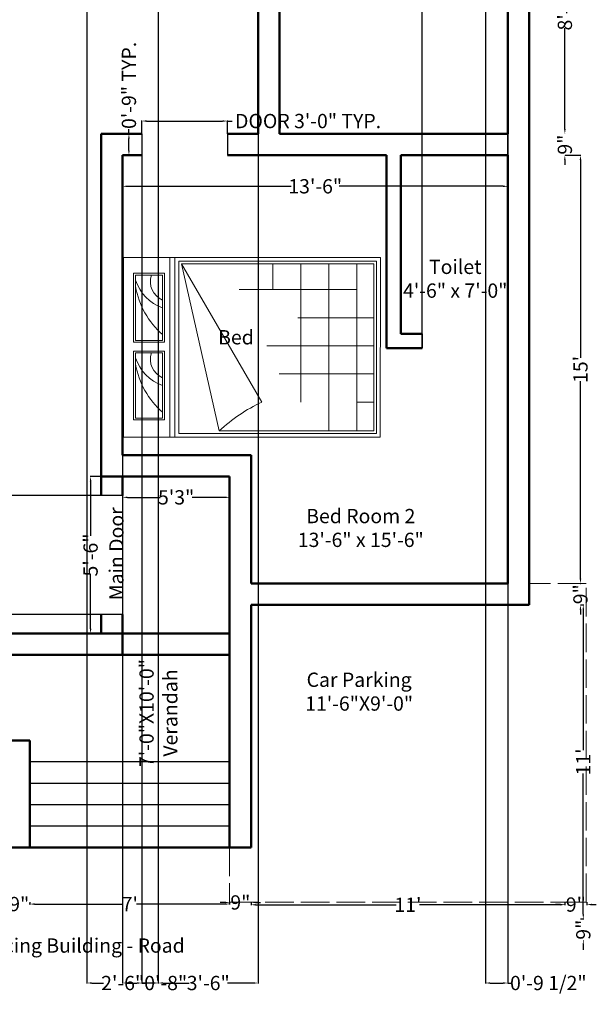
# Model space of a CAD drawing. Units: inches. Extents: x 35 to 505, y 81 to 785.
# Tile 2 of 3: x 224 to 466, y 81 to 495. Entities that reach past the tile are written whole.
import ezdxf

# ---------------------------------------------------------------- set-up
doc = ezdxf.new("R2010")
doc.units = ezdxf.units.IN
doc.header["$MEASUREMENT"] = 0
doc.linetypes.add('ACAD_ISO02W100', pattern=[15, 12, -3])
for name, color, linetype, lineweight in [('A-ANNO-DIMS', 2, 'Continuous', 13), ('A-ANNO-TEXT', 7, 'Continuous', 18), ('A-AREA-IDEN', 7, 'Continuous', 20), ('A-DOOR', 3, 'Continuous', 30), ('A-FLOR-STRS', 7, 'Continuous', 25), ('A-FURN', 6, 'Continuous', 18), ('A-WALL', 7, 'Continuous', 50), ('C-PKNG', 8, 'ACAD_ISO02W100', 18)]:
    doc.layers.add(name, color=color, linetype=linetype, lineweight=lineweight)
doc.styles.get("Standard").update_dxf_attribs({"font": 'arial.ttf'})
doc.dimstyles.get("Standard").update_dxf_attribs({"dimtxt": 6, "dimasz": 2, "dimexe": 0.18, "dimexo": 0.0625, "dimgap": 0.09, "dimtad": 0, "dimdec": 0, "dimzin": 0, "dimdsep": 46, "dimlunit": 4, "dimtxsty": 'Standard', "dimcen": 0.09, "dimadec": 0, "dimazin": 0, "dimtfac": 1, "dimtdec": 0, "dimtofl": 0, "dimtmove": 0, "dimatfit": 3, "dimfxl": 1, "dimtolj": 1, "dimtzin": 0, "dimarcsym": 0})

# ---------------------------------------------------------------- blocks, each defined once
blk = doc.blocks.new('*D19')
at = {"layer": 'A-ANNO-DIMS', "color": 0, "lineweight": -2, "transparency": 16777216}
for p, q in [((219.06, 124.18), (219.06, 123.2)), ((228.06, 124.18), (228.06, 123.2)), ((217.06, 123.38), (215.06, 123.38)), ((230.06, 123.38), (232.06, 123.38))]:
    blk.add_line(p, q, dxfattribs=at)
at = {"layer": 'A-ANNO-DIMS', "color": 0, "transparency": 16777216}
for points in [[(217.06, 123.71), (217.06, 123.04), (219.06, 123.38)], [(230.06, 123.71), (230.06, 123.04), (228.06, 123.38)]]:
    blk.add_solid(points, dxfattribs=at)
at = {"layer": 'Defpoints', "color": 0, "transparency": 16777216}
for p in [(219.06, 124.25), (228.06, 124.25), (219.06, 123.38)]:
    blk.add_point(p, dxfattribs=at)
at = {"layer": 'A-ANNO-DIMS', "color": 0, "transparency": 16777216, "insert": (223.56, 123.38), "char_height": 6, "attachment_point": 5}
blk.add_mtext('\\A1;9"', dxfattribs=at)
blk = doc.blocks.new('*D20')
at = {"layer": 'A-ANNO-DIMS', "color": 0, "lineweight": -2, "transparency": 16777216}
for p, q in [((312.06, 124.18), (312.06, 123.21)), ((228.06, 123.26), (228.06, 123.57)), ((230.06, 123.39), (267.23, 123.39)), ((310.06, 123.39), (272.88, 123.39))]:
    blk.add_line(p, q, dxfattribs=at)
at = {"layer": 'A-ANNO-DIMS', "color": 0, "transparency": 16777216}
for points in [[(230.06, 123.73), (230.06, 123.06), (228.06, 123.39)], [(310.06, 123.73), (310.06, 123.06), (312.06, 123.39)]]:
    blk.add_solid(points, dxfattribs=at)
at = {"layer": 'Defpoints', "color": 0, "transparency": 16777216}
for p in [(312.06, 124.25), (228.06, 123.2), (312.06, 123.39)]:
    blk.add_point(p, dxfattribs=at)
at = {"layer": 'A-ANNO-DIMS', "color": 0, "transparency": 16777216, "insert": (270.06, 123.39), "char_height": 6, "attachment_point": 5}
blk.add_mtext("\\A1;7'", dxfattribs=at)
blk = doc.blocks.new('*D21')
at = {"layer": 'A-ANNO-DIMS', "color": 0, "lineweight": -2, "transparency": 16777216}
for p, q in [((312.06, 123.45), (312.06, 124.24)), ((321.06, 124.18), (321.06, 123.88)), ((310.06, 124.06), (308.06, 124.06)), ((323.06, 124.06), (325.06, 124.06))]:
    blk.add_line(p, q, dxfattribs=at)
at = {"layer": 'A-ANNO-DIMS', "color": 0, "transparency": 16777216}
for points in [[(310.06, 124.39), (310.06, 123.73), (312.06, 124.06)], [(323.06, 124.39), (323.06, 123.73), (321.06, 124.06)]]:
    blk.add_solid(points, dxfattribs=at)
at = {"layer": 'Defpoints', "color": 0, "transparency": 16777216}
for p in [(321.06, 124.25), (312.06, 123.39), (321.06, 124.06)]:
    blk.add_point(p, dxfattribs=at)
at = {"layer": 'A-ANNO-DIMS', "color": 0, "transparency": 16777216, "insert": (316.56, 124.06), "char_height": 6, "attachment_point": 5}
blk.add_mtext('\\A1;9"', dxfattribs=at)
blk = doc.blocks.new('*D25')
at = {"layer": 'A-ANNO-DIMS', "color": 0, "lineweight": -2, "transparency": 16777216}
for p, q in [((453.12, 552.11), (453.24, 552.11)), ((453.06, 550.11), (453.06, 507.68)), ((453.06, 449.11), (453.06, 491.54)), ((453.12, 447.11), (453.24, 447.11))]:
    blk.add_line(p, q, dxfattribs=at)
at = {"layer": 'A-ANNO-DIMS', "color": 0, "transparency": 16777216}
for points in [[(452.72, 550.11), (453.39, 550.11), (453.06, 552.11)], [(452.72, 449.11), (453.39, 449.11), (453.06, 447.11)]]:
    blk.add_solid(points, dxfattribs=at)
at = {"layer": 'Defpoints', "color": 0, "transparency": 16777216}
for p in [(453.06, 552.11), (453.06, 447.11), (453.06, 447.11)]:
    blk.add_point(p, dxfattribs=at)
at = {"layer": 'A-ANNO-DIMS', "color": 0, "transparency": 16777216, "insert": (453.06, 499.61), "char_height": 6, "attachment_point": 5, "rotation": 90}
blk.add_mtext('\\A1;8\'-9"', dxfattribs=at)
blk = doc.blocks.new('*D26')
at = {"layer": 'A-ANNO-DIMS', "color": 0, "lineweight": -2, "transparency": 16777216}
for p, q in [((453.06, 449.11), (453.06, 451.11)), ((453.12, 447.11), (453.24, 447.11)), ((453.06, 436.11), (453.06, 434.11)), ((453.12, 438.11), (453.24, 438.11))]:
    blk.add_line(p, q, dxfattribs=at)
at = {"layer": 'A-ANNO-DIMS', "color": 0, "transparency": 16777216}
for points in [[(452.72, 449.11), (453.39, 449.11), (453.06, 447.11)], [(452.72, 436.11), (453.39, 436.11), (453.06, 438.11)]]:
    blk.add_solid(points, dxfattribs=at)
at = {"layer": 'Defpoints', "color": 0, "transparency": 16777216}
for p in [(453.06, 447.11), (453.06, 438.11), (453.06, 438.11)]:
    blk.add_point(p, dxfattribs=at)
at = {"layer": 'A-ANNO-DIMS', "color": 0, "transparency": 16777216, "insert": (453.06, 442.61), "char_height": 6, "attachment_point": 5, "rotation": 90}
blk.add_mtext('\\A1;9"', dxfattribs=at)
blk = doc.blocks.new('*D27')
at = {"layer": 'A-ANNO-DIMS', "color": 0, "lineweight": -2, "transparency": 16777216}
for p, q in [((453.12, 438.11), (459.8, 438.11)), ((459.62, 436.11), (459.62, 353.01)), ((459.62, 260.11), (459.62, 343.21)), ((459.69, 258.11), (459.8, 258.11))]:
    blk.add_line(p, q, dxfattribs=at)
at = {"layer": 'A-ANNO-DIMS', "color": 0, "transparency": 16777216}
for points in [[(459.29, 436.11), (459.96, 436.11), (459.62, 438.11)], [(459.29, 260.11), (459.96, 260.11), (459.62, 258.11)]]:
    blk.add_solid(points, dxfattribs=at)
at = {"layer": 'Defpoints', "color": 0, "transparency": 16777216}
for p in [(453.06, 438.11), (459.62, 258.11), (459.62, 258.11)]:
    blk.add_point(p, dxfattribs=at)
at = {"layer": 'A-ANNO-DIMS', "color": 0, "transparency": 16777216, "insert": (459.62, 348.11), "char_height": 6, "attachment_point": 5, "rotation": 90}
blk.add_mtext("\\A1;15'", dxfattribs=at)
blk = doc.blocks.new('*D28')
at = {"layer": 'A-ANNO-DIMS', "color": 0, "lineweight": -2, "transparency": 16777216}
for p, q in [((459.62, 260.11), (459.62, 262.11)), ((459.69, 258.11), (459.8, 258.11)), ((459.69, 249.11), (459.8, 249.11)), ((459.62, 247.11), (459.62, 245.11))]:
    blk.add_line(p, q, dxfattribs=at)
at = {"layer": 'A-ANNO-DIMS', "color": 0, "transparency": 16777216}
for points in [[(459.29, 260.11), (459.96, 260.11), (459.62, 258.11)], [(459.29, 247.11), (459.96, 247.11), (459.62, 249.11)]]:
    blk.add_solid(points, dxfattribs=at)
at = {"layer": 'Defpoints', "color": 0, "transparency": 16777216}
for p in [(459.62, 258.11), (459.62, 249.11), (459.62, 249.11)]:
    blk.add_point(p, dxfattribs=at)
at = {"layer": 'A-ANNO-DIMS', "color": 0, "transparency": 16777216, "insert": (459.62, 253.61), "char_height": 6, "attachment_point": 5, "rotation": 90}
blk.add_mtext('\\A1;9"', dxfattribs=at)
blk = doc.blocks.new('*D29')
at = {"layer": 'A-ANNO-DIMS', "color": 0, "lineweight": -2, "transparency": 16777216}
for p, q in [((459.69, 249.11), (460.99, 249.11)), ((460.81, 247.11), (460.81, 188.01)), ((460.81, 119.11), (460.81, 178.21)), ((459.69, 117.11), (460.99, 117.11))]:
    blk.add_line(p, q, dxfattribs=at)
at = {"layer": 'A-ANNO-DIMS', "color": 0, "transparency": 16777216}
for points in [[(460.47, 247.11), (461.14, 247.11), (460.81, 249.11)], [(460.47, 119.11), (461.14, 119.11), (460.81, 117.11)]]:
    blk.add_solid(points, dxfattribs=at)
at = {"layer": 'Defpoints', "color": 0, "transparency": 16777216}
for p in [(459.62, 249.11), (459.62, 117.11), (460.81, 117.11)]:
    blk.add_point(p, dxfattribs=at)
at = {"layer": 'A-ANNO-DIMS', "color": 0, "transparency": 16777216, "insert": (460.81, 183.11), "char_height": 6, "attachment_point": 5, "rotation": 90}
blk.add_mtext("\\A1;11'", dxfattribs=at)
blk = doc.blocks.new('*D30')
at = {"layer": 'A-ANNO-DIMS', "color": 0, "lineweight": -2, "transparency": 16777216}
for p, q in [((460.81, 119.11), (460.81, 121.11)), ((460.87, 117.11), (460.99, 117.11)), ((460.87, 108.11), (460.99, 108.11)), ((460.81, 106.11), (460.81, 104.11))]:
    blk.add_line(p, q, dxfattribs=at)
at = {"layer": 'A-ANNO-DIMS', "color": 0, "transparency": 16777216}
for points in [[(460.47, 119.11), (461.14, 119.11), (460.81, 117.11)], [(460.47, 106.11), (461.14, 106.11), (460.81, 108.11)]]:
    blk.add_solid(points, dxfattribs=at)
at = {"layer": 'Defpoints', "color": 0, "transparency": 16777216}
for p in [(460.81, 117.11), (460.81, 108.11), (460.81, 108.11)]:
    blk.add_point(p, dxfattribs=at)
at = {"layer": 'A-ANNO-DIMS', "color": 0, "transparency": 16777216, "insert": (460.81, 112.61), "char_height": 6, "attachment_point": 5, "rotation": 90}
blk.add_mtext('\\A1;9"', dxfattribs=at)
blk = doc.blocks.new('*D31')
at = {"layer": 'A-ANNO-DIMS', "color": 0, "lineweight": -2, "transparency": 16777216}
for p, q in [((267.06, 438.05), (267.06, 424.9)), ((429.06, 438.05), (429.06, 424.9)), ((269.06, 425.08), (337.94, 425.08)), ((427.06, 425.08), (358.17, 425.08))]:
    blk.add_line(p, q, dxfattribs=at)
at = {"layer": 'A-ANNO-DIMS', "color": 0, "transparency": 16777216}
for points in [[(269.06, 425.41), (269.06, 424.74), (267.06, 425.08)], [(427.06, 425.41), (427.06, 424.74), (429.06, 425.08)]]:
    blk.add_solid(points, dxfattribs=at)
at = {"layer": 'Defpoints', "color": 0, "transparency": 16777216}
for p in [(267.06, 438.11), (429.06, 438.11), (429.06, 425.08)]:
    blk.add_point(p, dxfattribs=at)
at = {"layer": 'A-ANNO-DIMS', "color": 0, "transparency": 16777216, "insert": (348.06, 425.08), "char_height": 6, "attachment_point": 5}
blk.add_mtext('\\A1;13\'-6"', dxfattribs=at)
blk = doc.blocks.new('*D32')
at = {"layer": 'A-ANNO-DIMS', "color": 0, "lineweight": -2, "transparency": 16777216}
for p, q in [((257.99, 303.11), (253.38, 303.11)), ((253.56, 301.11), (253.56, 278.17)), ((253.56, 239.11), (253.56, 262.04)), ((257.99, 237.11), (253.38, 237.11))]:
    blk.add_line(p, q, dxfattribs=at)
at = {"layer": 'A-ANNO-DIMS', "color": 0, "transparency": 16777216}
for points in [[(253.23, 301.11), (253.89, 301.11), (253.56, 303.11)], [(253.23, 239.11), (253.89, 239.11), (253.56, 237.11)]]:
    blk.add_solid(points, dxfattribs=at)
at = {"layer": 'Defpoints', "color": 0, "transparency": 16777216}
for p in [(253.56, 303.11), (258.06, 303.11), (258.06, 237.11)]:
    blk.add_point(p, dxfattribs=at)
at = {"layer": 'A-ANNO-DIMS', "color": 0, "transparency": 16777216, "insert": (253.56, 270.11), "char_height": 6, "attachment_point": 5, "rotation": 90}
blk.add_mtext('\\A1;5\'-6"', dxfattribs=at)
blk = doc.blocks.new('*D33')
at = {"layer": 'A-ANNO-DIMS', "color": 0, "lineweight": -2, "transparency": 16777216}
for p, q in [((321.06, 124.18), (321.06, 122.91)), ((453.06, 124.18), (453.06, 122.91)), ((323.06, 123.09), (382.16, 123.09)), ((451.06, 123.09), (391.96, 123.09))]:
    blk.add_line(p, q, dxfattribs=at)
at = {"layer": 'A-ANNO-DIMS', "color": 0, "transparency": 16777216}
for points in [[(323.06, 123.43), (323.06, 122.76), (321.06, 123.09)], [(451.06, 123.43), (451.06, 122.76), (453.06, 123.09)]]:
    blk.add_solid(points, dxfattribs=at)
at = {"layer": 'Defpoints', "color": 0, "transparency": 16777216}
for p in [(321.06, 124.25), (453.06, 124.25), (453.06, 123.09)]:
    blk.add_point(p, dxfattribs=at)
at = {"layer": 'A-ANNO-DIMS', "color": 0, "transparency": 16777216, "insert": (387.06, 123.09), "char_height": 6, "attachment_point": 5}
blk.add_mtext("\\A1;11'", dxfattribs=at)
blk = doc.blocks.new('*D34')
at = {"layer": 'A-ANNO-DIMS', "color": 0, "lineweight": -2, "transparency": 16777216}
for p, q in [((453.06, 124.18), (453.06, 122.99)), ((462.29, 124.18), (462.29, 122.99)), ((451.06, 123.17), (449.06, 123.17)), ((464.29, 123.17), (466.29, 123.17))]:
    blk.add_line(p, q, dxfattribs=at)
at = {"layer": 'A-ANNO-DIMS', "color": 0, "transparency": 16777216}
for points in [[(451.06, 123.51), (451.06, 122.84), (453.06, 123.17)], [(464.29, 123.51), (464.29, 122.84), (462.29, 123.17)]]:
    blk.add_solid(points, dxfattribs=at)
at = {"layer": 'Defpoints', "color": 0, "transparency": 16777216}
for p in [(453.06, 124.25), (462.29, 124.25), (462.29, 123.17)]:
    blk.add_point(p, dxfattribs=at)
at = {"layer": 'A-ANNO-DIMS', "color": 0, "transparency": 16777216, "insert": (457.68, 123.17), "char_height": 6, "attachment_point": 5}
blk.add_mtext('\\A1;9"', dxfattribs=at)
blk = doc.blocks.new('*D35')
at = {"layer": 'A-ANNO-DIMS', "color": 0, "lineweight": -2, "transparency": 16777216}
for p, q in [((267.06, 303.05), (267.06, 294.16)), ((312.06, 303.05), (312.06, 294.16)), ((269.06, 294.34), (282.89, 294.34)), ((310.06, 294.34), (296.23, 294.34))]:
    blk.add_line(p, q, dxfattribs=at)
at = {"layer": 'A-ANNO-DIMS', "color": 0, "transparency": 16777216}
for points in [[(269.06, 294.67), (269.06, 294.01), (267.06, 294.34)], [(310.06, 294.67), (310.06, 294.01), (312.06, 294.34)]]:
    blk.add_solid(points, dxfattribs=at)
at = {"layer": 'Defpoints', "color": 0, "transparency": 16777216}
for p in [(267.06, 303.11), (312.06, 303.11), (312.06, 294.34)]:
    blk.add_point(p, dxfattribs=at)
at = {"layer": 'A-ANNO-DIMS', "color": 0, "transparency": 16777216, "insert": (289.56, 294.34), "char_height": 6, "attachment_point": 5}
blk.add_mtext('\\A1;5\'3"', dxfattribs=at)
blk = doc.blocks.new('bed')
for p, q in [((309.37, 914.01), (309.37, 1021.97)), ((309.37, 1021.97), (384.97, 1021.97)), ((384.97, 1021.97), (384.97, 913.97)), ((316.65, 1017.78), (345.65, 1017.78)), ((316.65, 1004.77), (316.65, 1017.78)), ((317.46, 1016.97), (344.84, 1016.97)), ((317.46, 1005.58), (317.46, 1016.97)), ((344.84, 1016.97), (344.84, 1005.58)), ((345.65, 1017.78), (345.65, 1004.77)), ((349.3, 1017.78), (378.3, 1017.78)), ((349.3, 1004.77), (349.3, 1017.78)), ((350.11, 1016.97), (377.49, 1016.97)), ((350.11, 1005.58), (350.11, 1016.97)), ((377.49, 1016.97), (377.49, 1005.58)), ((378.3, 1017.78), (378.3, 1004.77)), ((309.37, 1002.53), (384.97, 1002.53)), ((345.65, 1004.77), (316.65, 1004.77)), ((344.84, 1005.58), (317.46, 1005.58)), ((378.3, 1004.77), (349.3, 1004.77)), ((377.49, 1005.58), (350.11, 1005.58)), ((309.37, 1000.37), (384.97, 1000.37)), ((310.99, 998.75), (383.35, 998.75)), ((310.99, 915.59), (310.99, 998.75)), ((382.27, 997.67), (312.07, 981.73)), ((382.27, 997.67), (324.17, 963.79)), ((382.27, 997.67), (382.27, 916.67)), ((383.35, 998.75), (383.35, 915.59)), ((312.07, 916.67), (312.07, 981.73)), ((371.46, 923.83), (371.46, 973.35)), ((347.84, 916.67), (347.84, 961.71)), ((336.02, 916.67), (336.02, 956.58)), ((371.46, 959.27), (382.27, 959.27)), ((359.65, 916.67), (359.65, 948.66)), ((324.21, 947.45), (382.27, 947.45)), ((312.07, 935.64), (382.27, 935.64)), ((312.07, 923.83), (382.27, 923.83)), ((324.21, 916.67), (324.21, 923.83)), ((383.35, 915.59), (310.99, 915.59)), ((382.27, 916.67), (312.07, 916.67)), ((384.97, 913.97), (309.37, 914.01))]:
    blk.add_line(p, q)
for centre, radius, start, end in [((346.35, 982.33), 35.21, 100.2734, 138.6774), ((348.52, 999.48), 18.4, 108.0489, 160.6348), ((378.99, 982.33), 35.21, 100.2734, 138.6774), ((381.16, 999.48), 18.4, 108.0489, 160.6348), ((342.22, 1002.22), 8.48, 71.9504, 156.6806), ((374.86, 1002.22), 8.48, 71.9504, 156.6806), ((263.08, 935.62), 67.27, 24.7582, 43.2711)]:
    blk.add_arc(centre, radius, start, end)
blk = doc.blocks.new('DOOR-36-JAMBS')
for p, q in [((0, 9), (0, 0)), ((36, 9), (36, 0))]:
    blk.add_line(p, q)
blk = doc.blocks.new('*D46')
at = {"layer": 'A-ANNO-DIMS', "color": 0, "lineweight": -2, "transparency": 16777216}
for p, q in [((275.09, 447.17), (275.09, 452.69)), ((277.09, 452.51), (309.09, 452.51)), ((311.09, 447.17), (311.09, 452.69)), ((311.09, 452.51), (313.09, 452.51))]:
    blk.add_line(p, q, dxfattribs=at)
at = {"layer": 'A-ANNO-DIMS', "color": 0, "transparency": 16777216}
for points in [[(277.09, 452.84), (277.09, 452.18), (275.09, 452.51)], [(309.09, 452.84), (309.09, 452.18), (311.09, 452.51)]]:
    blk.add_solid(points, dxfattribs=at)
at = {"layer": 'Defpoints', "color": 0, "transparency": 16777216}
for p in [(311.09, 452.51), (275.09, 447.11), (311.09, 447.11)]:
    blk.add_point(p, dxfattribs=at)
at = {"layer": 'A-ANNO-DIMS', "color": 0, "transparency": 16777216, "insert": (345.06, 452.51), "char_height": 6, "attachment_point": 5}
blk.add_mtext('\\A1;DOOR 3\'-0" TYP.', dxfattribs=at)
blk = doc.blocks.new('*D47')
at = {"layer": 'A-ANNO-DIMS', "color": 0, "lineweight": -2, "transparency": 16777216}
for p, q in [((275.03, 447.11), (269.51, 447.11)), ((269.69, 447.11), (269.69, 449.11)), ((269.69, 440.11), (269.69, 445.11)), ((275.03, 438.11), (269.51, 438.11))]:
    blk.add_line(p, q, dxfattribs=at)
at = {"layer": 'A-ANNO-DIMS', "color": 0, "transparency": 16777216}
for points in [[(269.36, 445.11), (270.03, 445.11), (269.69, 447.11)], [(269.36, 440.11), (270.03, 440.11), (269.69, 438.11)]]:
    blk.add_solid(points, dxfattribs=at)
at = {"layer": 'Defpoints', "color": 0, "transparency": 16777216}
for p in [(269.69, 447.11), (275.09, 447.11), (275.09, 438.11)]:
    blk.add_point(p, dxfattribs=at)
at = {"layer": 'A-ANNO-DIMS', "color": 0, "transparency": 16777216, "insert": (269.69, 467.49), "char_height": 6, "attachment_point": 5, "rotation": 90}
blk.add_mtext('\\A1;0\'-9" TYP.', dxfattribs=at)
blk = doc.blocks.new('*D58')
at = {"layer": 'A-ANNO-DIMS', "color": 0, "lineweight": -2, "transparency": 16777216}
for p, q in [((257.99, 295.11), (43.83, 295.11)), ((44.01, 293.11), (44.01, 278.29)), ((44.01, 247.11), (44.01, 261.92)), ((257.99, 245.11), (43.83, 245.11))]:
    blk.add_line(p, q, dxfattribs=at)
at = {"layer": 'A-ANNO-DIMS', "color": 0, "transparency": 16777216}
for points in [[(43.67, 293.11), (44.34, 293.11), (44.01, 295.11)], [(43.67, 247.11), (44.34, 247.11), (44.01, 245.11)]]:
    blk.add_solid(points, dxfattribs=at)
at = {"layer": 'Defpoints', "color": 0, "transparency": 16777216}
for p in [(44.01, 295.11), (258.06, 295.11), (258.06, 245.11)]:
    blk.add_point(p, dxfattribs=at)
at = {"layer": 'A-ANNO-DIMS', "color": 0, "transparency": 16777216, "insert": (44.01, 270.11), "char_height": 6, "attachment_point": 5, "rotation": 90}
blk.add_mtext('\\A1;4\'-2"', dxfattribs=at)
blk = doc.blocks.new('*D59')
at = {"layer": 'A-ANNO-DIMS', "color": 0, "lineweight": -2, "transparency": 16777216}
for p, q in [((267.06, 438.05), (267.06, 90.02)), ((275.09, 438.05), (275.09, 90.02)), ((269.06, 90.2), (273.09, 90.2)), ((275.09, 90.2), (277.09, 90.2))]:
    blk.add_line(p, q, dxfattribs=at)
at = {"layer": 'A-ANNO-DIMS', "color": 0, "transparency": 16777216}
for points in [[(269.06, 90.53), (269.06, 89.86), (267.06, 90.2)], [(273.09, 90.53), (273.09, 89.86), (275.09, 90.2)]]:
    blk.add_solid(points, dxfattribs=at)
at = {"layer": 'Defpoints', "color": 0, "transparency": 16777216}
for p in [(267.06, 438.11), (275.09, 438.11), (275.09, 90.2)]:
    blk.add_point(p, dxfattribs=at)
at = {"layer": 'A-ANNO-DIMS', "color": 0, "transparency": 16777216, "insert": (285.16, 90.2), "char_height": 6, "attachment_point": 5}
blk.add_mtext('\\A1;0\'-8"', dxfattribs=at)
blk = doc.blocks.new('*D62')
at = {"layer": 'A-ANNO-DIMS', "color": 0, "lineweight": -2, "transparency": 16777216}
for p, q in [((252.06, 561.05), (252.06, 90.02)), ((282.06, 561.05), (282.06, 90.02)), ((254.06, 90.2), (258.94, 90.2)), ((280.06, 90.2), (275.17, 90.2))]:
    blk.add_line(p, q, dxfattribs=at)
at = {"layer": 'A-ANNO-DIMS', "color": 0, "transparency": 16777216}
for points in [[(254.06, 90.53), (254.06, 89.86), (252.06, 90.2)], [(280.06, 90.53), (280.06, 89.86), (282.06, 90.2)]]:
    blk.add_solid(points, dxfattribs=at)
at = {"layer": 'Defpoints', "color": 0, "transparency": 16777216}
for p in [(252.06, 561.11), (282.06, 561.11), (282.06, 90.2)]:
    blk.add_point(p, dxfattribs=at)
at = {"layer": 'A-ANNO-DIMS', "color": 0, "transparency": 16777216, "insert": (267.06, 90.2), "char_height": 6, "attachment_point": 5}
blk.add_mtext('\\A1;2\'-6"', dxfattribs=at)
blk = doc.blocks.new('*D63')
at = {"layer": 'A-ANNO-DIMS', "color": 0, "lineweight": -2, "transparency": 16777216}
for p, q in [((282.06, 552.05), (282.06, 90.02)), ((324.06, 552.05), (324.06, 90.02)), ((284.06, 90.2), (294.99, 90.2)), ((322.06, 90.2), (311.12, 90.2))]:
    blk.add_line(p, q, dxfattribs=at)
at = {"layer": 'A-ANNO-DIMS', "color": 0, "transparency": 16777216}
for points in [[(284.06, 90.53), (284.06, 89.86), (282.06, 90.2)], [(322.06, 90.53), (322.06, 89.86), (324.06, 90.2)]]:
    blk.add_solid(points, dxfattribs=at)
at = {"layer": 'Defpoints', "color": 0, "transparency": 16777216}
for p in [(282.06, 552.11), (324.06, 552.11), (324.06, 90.2)]:
    blk.add_point(p, dxfattribs=at)
at = {"layer": 'A-ANNO-DIMS', "color": 0, "transparency": 16777216, "insert": (303.06, 90.2), "char_height": 6, "attachment_point": 5}
blk.add_mtext('\\A1;3\'-6"', dxfattribs=at)
blk = doc.blocks.new('*D65')
at = {"layer": 'A-ANNO-DIMS', "color": 0, "lineweight": -2, "transparency": 16777216}
for p, q in [((393.06, 357.17), (393.06, 781.34)), ((395.06, 781.16), (402.99, 781.16)), ((427.06, 781.16), (419.12, 781.16)), ((429.06, 258.17), (429.06, 781.34))]:
    blk.add_line(p, q, dxfattribs=at)
at = {"layer": 'A-ANNO-DIMS', "color": 0, "transparency": 16777216}
for points in [[(395.06, 781.49), (395.06, 780.83), (393.06, 781.16)], [(427.06, 781.49), (427.06, 780.83), (429.06, 781.16)]]:
    blk.add_solid(points, dxfattribs=at)
at = {"layer": 'Defpoints', "color": 0, "transparency": 16777216}
for p in [(429.06, 781.16), (393.06, 357.11), (429.06, 258.11)]:
    blk.add_point(p, dxfattribs=at)
at = {"layer": 'A-ANNO-DIMS', "color": 0, "transparency": 16777216, "insert": (411.06, 781.16), "char_height": 6, "attachment_point": 5}
blk.add_mtext('\\A1;3\'-0"', dxfattribs=at)
blk = doc.blocks.new('*D67')
at = {"layer": 'A-ANNO-DIMS', "color": 0, "lineweight": -2, "transparency": 16777216}
for p, q in [((419.64, 645.05), (419.64, 90.02)), ((429.06, 645.05), (429.06, 90.02)), ((421.64, 90.2), (427.06, 90.2)), ((429.06, 90.2), (431.06, 90.2))]:
    blk.add_line(p, q, dxfattribs=at)
at = {"layer": 'A-ANNO-DIMS', "color": 0, "transparency": 16777216}
for points in [[(421.64, 90.53), (421.64, 89.86), (419.64, 90.2)], [(427.06, 90.53), (427.06, 89.86), (429.06, 90.2)]]:
    blk.add_solid(points, dxfattribs=at)
at = {"layer": 'Defpoints', "color": 0, "transparency": 16777216}
for p in [(419.64, 645.11), (429.06, 645.11), (429.06, 90.2)]:
    blk.add_point(p, dxfattribs=at)
at = {"layer": 'A-ANNO-DIMS', "color": 0, "transparency": 16777216, "insert": (446.11, 90.2), "char_height": 6, "attachment_point": 5}
blk.add_mtext('\\A1;0\'-9 1/2"', dxfattribs=at)

msp = doc.modelspace()

# ---------------------------------------------------------------- linework, layer by layer
at = {"layer": 'A-DOOR'}
for p, q in [((393.06, 363.11), (393.06, 357.11)), ((267.06, 295.11), (258.06, 295.11)), ((267.06, 245.11), (258.06, 245.11))]:
    msp.add_line(p, q, dxfattribs=at)
at = {"layer": 'A-FLOR-STRS'}
for p, q in [((312.06, 183.11), (228.06, 183.11)), ((312.06, 174.11), (228.06, 174.11)), ((312.06, 165.11), (228.06, 165.11)), ((312.06, 156.11), (228.06, 156.11))]:
    msp.add_line(p, q, dxfattribs=at)
at = {"layer": 'A-WALL'}
for p, q in [((438.06, 747.11), (438.06, 249.11)), ((324.06, 552.11), (324.06, 447.11)), ((333.06, 552.11), (333.06, 447.11)), ((429.06, 552.11), (429.06, 447.11)), ((258.06, 447.11), (258.06, 295.11)), ((275.09, 447.11), (258.06, 447.11)), ((324.06, 447.11), (311.09, 447.11)), ((429.06, 447.11), (333.06, 447.11)), ((267.06, 438.11), (267.06, 312.11)), ((275.09, 438.11), (267.06, 438.11)), ((378.06, 438.11), (311.09, 438.11)), ((378.06, 438.11), (378.06, 357.11)), ((429.06, 438.11), (384.06, 438.11)), ((384.06, 438.11), (384.06, 363.11)), ((429.06, 438.11), (429.06, 258.11)), ((393.06, 363.11), (384.06, 363.11)), ((393.06, 357.11), (378.06, 357.11)), ((321.06, 312.11), (267.06, 312.11)), ((321.06, 312.11), (321.06, 258.11)), ((312.06, 303.11), (258.06, 303.11)), ((267.06, 303.11), (267.06, 295.11)), ((312.06, 303.11), (312.06, 228.11)), ((429.06, 258.11), (321.06, 258.11)), ((438.06, 249.11), (321.06, 249.11)), ((321.06, 249.11), (321.06, 147.11)), ((258.06, 245.11), (258.06, 237.11)), ((267.06, 245.11), (267.06, 228.11)), ((258.06, 237.11), (87.06, 237.11)), ((312.06, 237.11), (258.06, 237.11)), ((312.06, 228.11), (219.06, 228.11)), ((312.06, 228.11), (312.06, 147.11)), ((228.06, 192.11), (219.06, 192.11)), ((228.06, 192.11), (228.06, 147.11)), ((321.06, 147.11), (78.06, 147.11))]:
    msp.add_line(p, q, dxfattribs=at)
at = {"layer": 'C-PKNG'}
msp.add_lwpolyline([(312.06, 147.11), (312.06, 124.25), (453.06, 124.25), (462.06, 124.25), (462.06, 258.11), (438.06, 258.11)], dxfattribs=at)

# ---------------------------------------------------------------- block references
at = {"layer": 'A-DOOR'}
msp.add_blockref('DOOR-36-JAMBS', (275.09, 438.11), dxfattribs=at)
at = {"layer": 'A-FURN', "rotation": 90}
msp.add_blockref('bed', (1289.43, 10.2), dxfattribs=at)

# ---------------------------------------------------------------- texts
at = {"layer": 'A-ANNO-TEXT', "char_height": 6, "attachment_point": 1}
for s, width, insert in [('Bed', 25.2815, (307.22, 364.63)), ('\\pxqc;South Facing Building - Road', 193.0111, (141.71, 108.95))]:
    msp.add_mtext_dynamic_manual_height_columns(s, width=width, gutter_width=30, heights=[0], dxfattribs=dict(at, insert=insert))
at = {"layer": 'A-ANNO-TEXT', "insert": (261.41, 237.89), "char_height": 6, "attachment_point": 1, "rotation": 90}
msp.add_mtext_dynamic_manual_height_columns('\\pxqc;Main Door', width=65.4821, gutter_width=30, heights=[0], dxfattribs=at)
at = {"layer": 'A-AREA-IDEN', "char_height": 6, "attachment_point": 1}
for s, width, insert in [('\\pxqc;Toilet\\P4\'-6" x 7\'-0"', 68.2568, (372.82, 394.23)), ('\\pxqc;Bed Room 2\\P13\'-6" x 15\'-6"', 80.6316, (326.91, 289.47)), ('\\pxqc;Car Parking\\P11\'-6"X9\'-0"', 126.7103, (303.17, 220.67))]:
    msp.add_mtext_dynamic_manual_height_columns(s, width=width, gutter_width=30, heights=[0], dxfattribs=dict(at, insert=insert))
at = {"layer": 'A-AREA-IDEN', "insert": (274.1, 142.51), "char_height": 6, "attachment_point": 1, "rotation": 90}
msp.add_mtext_dynamic_manual_height_columns('\\pxqc;7\'-0"X10\'-0"\\PVerandah', width=122.3347, gutter_width=30, heights=[0], dxfattribs=at)

# ---------------------------------------------------------------- dimensions: what is measured, and where the dimension line sits
at = {"layer": 'A-ANNO-DIMS'}
for base, p1, p2, override, picture, middle in [((429.06, 781.16), (393.06, 357.11), (429.06, 258.11), {"dimdec": 1, "dimlfac": 1, "dimrnd": 0, "dimzin": 1, "dimdsep": 46, "dimlunit": 4, "dimfrac": 2}, '*D65', (411.06, 781.16)), ((429.06, 90.2), (419.64, 645.11), (429.06, 645.11), {"dimdec": 1, "dimlfac": 1, "dimrnd": 0, "dimzin": 1, "dimdsep": 46, "dimlunit": 4, "dimfrac": 2}, '*D67', (446.11, 90.2)), ((282.06, 90.2), (252.06, 561.11), (282.06, 561.11), {"dimdec": 1, "dimlfac": 1, "dimrnd": 0, "dimzin": 1, "dimdsep": 46, "dimlunit": 4, "dimfrac": 2}, '*D62', (267.06, 90.2)), ((324.06, 90.2), (282.06, 552.11), (324.06, 552.11), {"dimdec": 1, "dimlfac": 1, "dimrnd": 0, "dimzin": 1, "dimdsep": 46, "dimlunit": 4, "dimfrac": 2}, '*D63', (303.06, 90.2)), ((429.06, 425.08), (267.06, 438.11), (429.06, 438.11), {"dimclrd": 0, "dimclre": 0, "dimclrt": 0}, '*D31', (348.06, 425.08)), ((275.09, 90.2), (267.06, 438.11), (275.09, 438.11), {"dimdec": 1, "dimlfac": 1, "dimrnd": 0, "dimzin": 1, "dimdsep": 46, "dimlunit": 4, "dimfrac": 2}, '*D59', (285.16, 90.2)), ((219.06, 123.38), (228.06, 124.25), (219.06, 124.25), {"dimclrd": 0, "dimclre": 0, "dimclrt": 0}, '*D19', (223.56, 123.38)), ((312.06, 123.39), (228.06, 123.2), (312.06, 124.25), {"dimclrd": 0, "dimclre": 0, "dimclrt": 0}, '*D20', (270.06, 123.39)), ((321.06, 124.06), (312.06, 123.39), (321.06, 124.25), {"dimclrd": 0, "dimclre": 0, "dimclrt": 0}, '*D21', (316.56, 124.06)), ((453.06, 123.09), (321.06, 124.25), (453.06, 124.25), {"dimclrd": 0, "dimclre": 0, "dimclrt": 0}, '*D33', (387.06, 123.09)), ((462.29, 123.17), (453.06, 124.25), (462.29, 124.25), {"dimclrd": 0, "dimclre": 0, "dimclrt": 0}, '*D34', (457.68, 123.17))]:
    dim = msp.add_linear_dim(base=base, p1=p1, p2=p2, dimstyle='Standard', override=override, dxfattribs=at)
    dim.commit()
    dim.dimension.update_dxf_attribs({"geometry": picture, "text_midpoint": middle})
for base, p1, p2, override, picture, middle in [((453.06, 447.11), (453.06, 552.11), (453.06, 447.11), {"dimclrd": 0, "dimclre": 0, "dimclrt": 0}, '*D25', (453.06, 499.61)), ((453.06, 438.11), (453.06, 447.11), (453.06, 438.11), {"dimclrd": 0, "dimclre": 0, "dimclrt": 0}, '*D26', (453.06, 442.61)), ((459.62, 258.11), (453.06, 438.11), (459.62, 258.11), {"dimclrd": 0, "dimclre": 0, "dimclrt": 0}, '*D27', (459.62, 348.11)), ((253.56, 303.11), (258.06, 237.11), (258.06, 303.11), {"dimclrd": 0, "dimclre": 0, "dimclrt": 0}, '*D32', (253.56, 270.11)), ((44.01, 295.11), (258.06, 245.11), (258.06, 295.11), {"dimdec": 1, "dimlfac": 1, "dimrnd": 0, "dimzin": 1, "dimdsep": 46, "dimlunit": 4, "dimfrac": 2}, '*D58', (44.01, 270.11)), ((459.62, 249.11), (459.62, 258.11), (459.62, 249.11), {"dimclrd": 0, "dimclre": 0, "dimclrt": 0}, '*D28', (459.62, 253.61)), ((460.81, 117.11), (459.62, 249.11), (459.62, 117.11), {"dimclrd": 0, "dimclre": 0, "dimclrt": 0}, '*D29', (460.81, 183.11)), ((460.81, 108.11), (460.81, 117.11), (460.81, 108.11), {"dimclrd": 0, "dimclre": 0, "dimclrt": 0}, '*D30', (460.81, 112.61))]:
    dim = msp.add_linear_dim(base=base, p1=p1, p2=p2, angle=90, dimstyle='Standard', override=override, dxfattribs=at)
    dim.commit()
    dim.dimension.update_dxf_attribs({"geometry": picture, "text_midpoint": middle})
dim = msp.add_linear_dim(base=(269.69, 447.11), p1=(275.09, 438.11), p2=(275.09, 447.11), angle=90, text='<> TYP.', dimstyle='Standard', override={"dimdec": 1, "dimlfac": 1, "dimrnd": 0, "dimzin": 1, "dimdsep": 46, "dimlunit": 4, "dimfrac": 2}, dxfattribs=at)
dim.commit()
dim.dimension.update_dxf_attribs({"geometry": '*D47', "text_midpoint": (269.69, 467.49)})
for base, p1, p2, text, override, picture, middle in [((311.09, 452.51), (275.09, 447.11), (311.09, 447.11), 'DOOR <> TYP.', {"dimdec": 1, "dimlfac": 1, "dimrnd": 0, "dimzin": 1, "dimdsep": 46, "dimlunit": 4, "dimfrac": 2}, '*D46', (345.06, 452.51)), ((312.06, 294.34), (267.06, 303.11), (312.06, 303.11), '5\'3"', {"dimclrd": 0, "dimclre": 0, "dimclrt": 0}, '*D35', (289.56, 294.34))]:
    dim = msp.add_linear_dim(base=base, p1=p1, p2=p2, text=text, dimstyle='Standard', override=override, dxfattribs=at)
    dim.commit()
    dim.dimension.update_dxf_attribs({"geometry": picture, "text_midpoint": middle})

doc.saveas('drawing.dxf')
